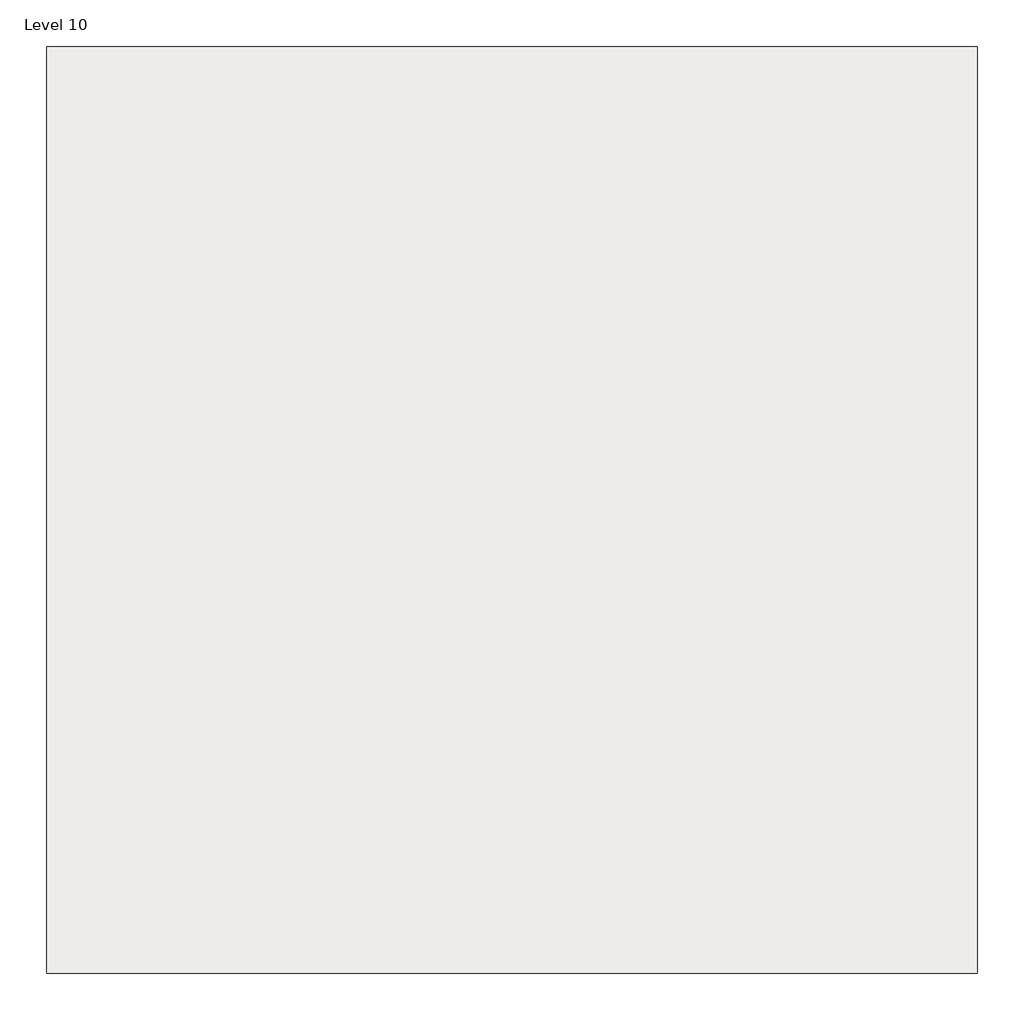
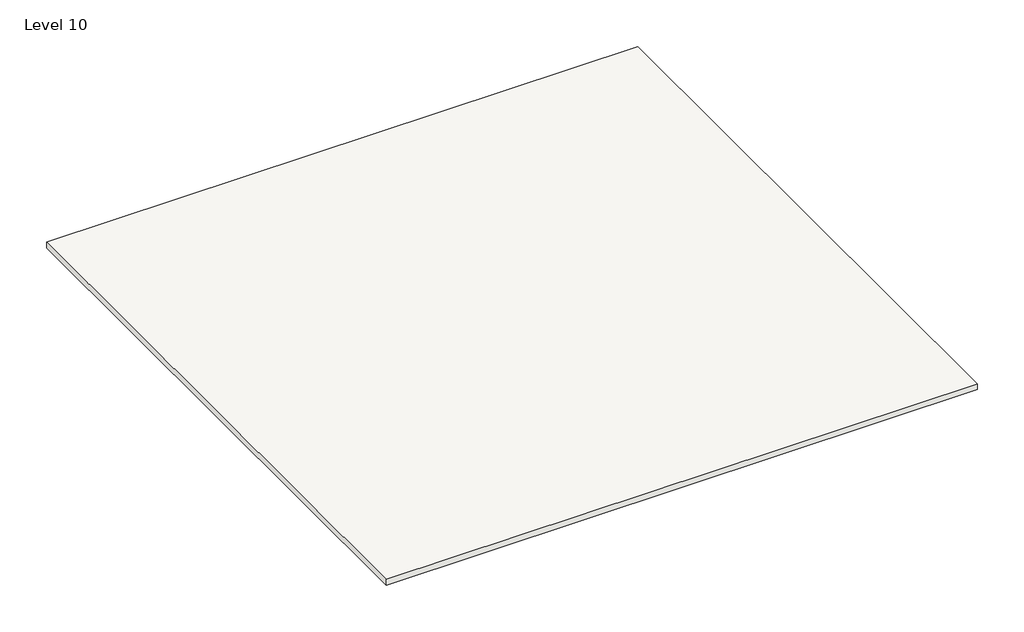
# One storey: 1 roof.
"""IFC4 building model written with IfcOpenShell, lengths in millimetres."""

from ifc_helpers import new_model, si_unit, frame, origin, place, context, project, spatial, polyline, outline, extrude, element, save

model = new_model("IFC4")

# Units and contexts
model_context = context("Model", 3, world=origin())
ifc_project = project(units=[si_unit("LENGTHUNIT", "METRE", prefix="MILLI")], contexts=[model_context])

# Site, building, storey
site = spatial("IfcSite", under=ifc_project)
building = spatial("IfcBuilding", under=site)
storey = spatial("IfcBuildingStorey", under=building, Name="Level 10", Elevation=16154.4)

# Roof
placement = place(None, origin())
element("IfcRoof", 1, ObjectType="Generic - 9\"", at=placement, inside=storey, context=model_context, shape_type="SweptSolid", body=[
    extrude(outline(polyline([(-8934.7629849, 17755.0995758), (12604.4370151, 17755.0995758), (12604.4370151, -3682.5004242), (-8934.7629849, -3682.5004242), (-8934.7629849, 17755.0995758)])), frame((0.0, 0.0, 16154.4), z_axis=(0.0, 0.0, 1.0), x_axis=(1.0, 0.0, 0.0)), (0.0, 0.0, 1.0), 228.6),
])

save(model, "model.ifc")

# Revit data of these elements
# Type "Generic - 9\""
#   Assembly Code = "B1020"
#   Layers, outside or top first: 0' - 9" no material (function 1)
# Element 1 (IfcRoof, "Generic - 9\"")
#   built-in parameter 1001705 = 53.75 (stored number, unit not read)
#   built-in parameter 1001710 = 33615
#   Phase Created = New Construction
#   Materials on its faces: "Default Roof"
# Materials
#   "Default Roof": colour RGB 88 101 114, transparency 0
